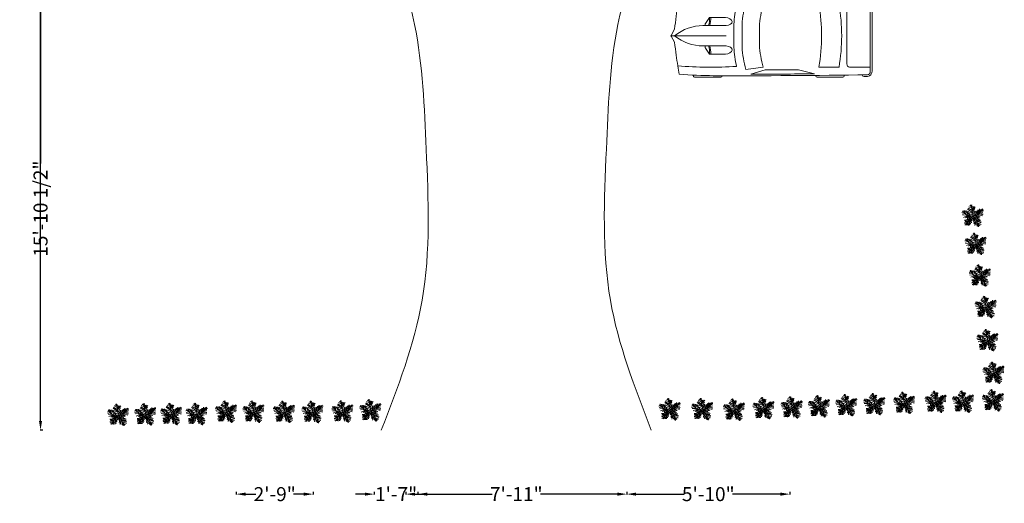
# Model space of a CAD drawing. Units: inches. Extents: x -81 to 380, y -521 to 79.
# Tile 1 of 5: x -81 to 342, y -521 to -313. Entities that reach past the tile are written whole.
import ezdxf

# ---------------------------------------------------------------- set-up
doc = ezdxf.new("R2010")
doc.units = ezdxf.units.IN
doc.header["$MEASUREMENT"] = 0
for name, color, linetype, lineweight in [('A-ANNO-DIMS', 2, 'Continuous', 18), ('C-ROAD-DRWY', 6, 'Continuous', 18), ('car', 33, 'Continuous', 18), ('trees', 3, 'Continuous', 13)]:
    doc.layers.add(name, color=color, linetype=linetype, lineweight=lineweight)
doc.styles.get("Standard").update_dxf_attribs({"font": 'arial.ttf'})
doc.dimstyles.get("Standard").update_dxf_attribs({"dimtxt": 6, "dimasz": 4, "dimexe": 0.18, "dimexo": 0.0625, "dimgap": 0.09, "dimtad": 0, "dimdec": 0, "dimzin": 0, "dimdsep": 46, "dimlunit": 3, "dimtxsty": 'Standard', "dimcen": 0.09, "dimclrd": 6, "dimclre": 6, "dimclrt": 2, "dimadec": 0, "dimazin": 0, "dimtfac": 1, "dimtdec": 0, "dimtofl": 0, "dimtmove": 0, "dimatfit": 3, "dimfxl": 1, "dimfxlon": 1, "dimtolj": 1, "dimtzin": 0, "dimarcsym": 0})

# ---------------------------------------------------------------- blocks, each defined once
blk = doc.blocks.new('*U4')
for p, q in [((-8.737, 47.138), (-17.069, 52.711)), ((-10.186, 53.64), (-13.084, 55.962)), ((0, 0), (-10.5, 57)), ((-9.099, 51.782), (-6.563, 55.962)), ((-7.65, 43.423), (-2.578, 49.46)), ((-47.498, 19.737), (-55.83, 18.344)), ((-40.615, 13.7), (-55.105, 10.913)), ((-31.5, 4.5), (-52.5, 25.5)), ((-33.37, 6.269), (-52.207, 5.34)), ((-48.585, 21.131), (-49.309, 29.026)), ((-28.299, 3.483), (-47.86, -5.805)), ((-43.513, 28.561), (-42.427, 15.558)), ((-38.442, 26.239), (-34.819, 7.663)), ((-21.416, 3.018), (-38.079, -8.128)), ((-35.544, 28.097), (-24.314, 3.947)), ((0, 0), (-31.5, 4.5)), ((-14.533, 2.09), (-30.834, 25.31)), ((-15.982, 2.09), (-30.11, -9.521)), ((-3.665, 19.273), (-27.574, 35.527)), ((-5.114, 28.097), (-24.676, 40.636)), ((-24.314, 23.917), (-2.941, 13.7)), ((0, 0), (-22.5, -19.5)), ((-7.288, 39.707), (-21.778, 46.673)), ((-6.563, 1.161), (-21.416, -8.128)), ((-20.691, 13.7), (-1.129, 4.876)), ((-5.839, 35.992), (4.667, 48.067)), ((-5.114, 27.632), (10.463, 46.673)), ((-2.941, 16.486), (8.652, 37.85)), ((-1.129, 6.734), (9.014, 26.704)), ((0, 0), (27, 9)), ((0, 0), (18, -22.5)), ((3.942, 1.625), (11.187, 24.381)), ((6.478, 1.625), (26.04, -8.592)), ((10.101, 3.483), (17.708, 26.239)), ((11.187, 3.483), (30.749, -5.805)), ((16.259, 5.805), (23.142, 31.348)), ((18.07, 5.805), (35.096, -3.483)), ((22.055, 7.198), (27.489, 32.277)), ((24.229, 7.663), (46.688, 1.625)), ((27, 9), (48, 36)), ((27.127, 9.056), (31.112, 35.992)), ((29.662, 12.307), (48.137, 6.269)), ((31.836, 30.883), (32.561, 16.486)), ((33.285, 16.486), (48.862, 10.913)), ((35.096, 32.741), (37.27, 22.524)), ((36.183, 19.737), (48.137, 17.88)), ((38.719, 34.134), (41.979, 28.561)), ((40.53, 25.775), (48.862, 24.846)), ((43.791, 29.954), (51.036, 30.883)), ((44.153, 36.456), (45.239, 32.741)), ((-17.431, -15.094), (-42.789, -18.809)), ((-28.299, -29.026), (-42.789, -31.348)), ((-24.314, -21.596), (-42.427, -22.06)), ((-30.834, -34.135), (-42.427, -35.528)), ((-34.457, -39.708), (-40.978, -42.494)), ((-26.849, -26.24), (-40.253, -25.775)), ((-22.5, -19.5), (-37.5, -45)), ((-32.646, -36.921), (-31.921, -44.352)), ((-15.257, -12.772), (-30.11, -12.772)), ((-29.023, -30.884), (-27.936, -43.887)), ((-25.038, -23.918), (-22.865, -45.281)), ((-20.691, -18.345), (-17.793, -44.352)), ((-6.563, -5.805), (-19.967, -9.985)), ((-17.069, -15.094), (-12.721, -40.172)), ((-13.446, -11.378), (-8.737, -32.741)), ((-9.461, -8.592), (-6.201, -23.453)), ((-4.752, -3.483), (-3.665, -14.629)), ((2.493, -3.019), (-1.491, -20.202)), ((1.769, -2.555), (24.229, -9.521)), ((5.029, -6.27), (2.131, -25.775)), ((9.014, -11.378), (3.58, -35.992)), ((14.085, -16.951), (6.478, -40.172)), ((7.565, -9.056), (32.198, -14.629)), ((18.07, -22.524), (8.289, -45.745)), ((12.274, -15.094), (36.907, -18.809)), ((20.244, -30.419), (15.897, -44.816)), ((16.259, -19.738), (36.183, -22.989)), ((18, -22.5), (27, -52.5)), ((18.433, -22.524), (40.53, -29.026)), ((19.157, -25.311), (38.719, -33.206)), ((22.78, -37.85), (19.519, -48.532)), ((21.331, -32.741), (39.081, -40.636)), ((22.78, -38.314), (34.372, -44.816)), ((24.591, -45.745), (23.142, -50.854)), ((24.591, -43.423), (30.749, -47.603)), ((26.764, -49.925), (28.213, -50.854))]:
    blk.add_line(p, q)
blk = doc.blocks.new('*U33')
for p, q in [((21.1, 37.41), (21.1, 36.83)), ((46.55, 38.89), (22.35, 38.89)), ((47.8, 37.39), (47.8, 37.41)), ((135.45, 37.07), (135.45, 37.41)), ((136.7, 38.89), (160.9, 38.89)), ((162.15, 37.41), (162.15, 36.77)), ((70.03, 31.54), (86.41, 29.35)), ((87.99, 31.87), (74.76, 35.92)), ((134.31, 35.6), (119.29, 31.78)), ((138.42, 29.35), (157.25, 29.35)), ((186.47, 29.35), (167.01, 29.35)), ((186.47, -33.5), (186.47, 33.5)), ((188.4, -32.76), (188.4, 32.76)), ((164.52, 26.39), (164.52, -26.39)), ((29.77, 9.51), (51.68, 9.51)), ((32.12, 9.51), (32.12, 11.15)), ((32.27, 11.63), (36.13, 17.17)), ((36.13, 17.17), (50.94, 17.17)), ((58.92, -10.77), (58.92, 10.77)), ((66.55, -10.53), (66.55, 10.53)), ((186.47, -10.53), (186.47, 10.53)), ((3.27, 6.13), (0.1, 0.41)), ((82.74, 8.5), (82.74, -8.5)), ((0, 0), (51.68, 0)), ((0.1, -0.41), (3.27, -6.13)), ((29.77, -9.51), (51.68, -9.51)), ((32.12, -9.51), (32.12, -11.15)), ((32.27, -11.63), (36.13, -17.17)), ((36.13, -17.17), (50.94, -17.17)), ((21.1, -37.41), (21.1, -36.83)), ((86.41, -29.35), (70.03, -31.54)), ((87.99, -31.87), (74.76, -35.92)), ((134.31, -35.6), (119.29, -31.78)), ((157.25, -29.35), (138.42, -29.35)), ((162.15, -37.41), (162.15, -36.77)), ((167.01, -29.35), (186.47, -29.35)), ((46.55, -38.89), (22.35, -38.89)), ((47.8, -37.39), (47.8, -37.41)), ((135.45, -37.07), (135.45, -37.41)), ((136.7, -38.89), (160.9, -38.89))]:
    blk.add_line(p, q)
for centre, major_axis, ratio, start_param, end_param in [((41.19, -490.86), (0, 528.23), 0.842304, 0.00281, 0.075598), ((22.35, 37.41), (0, -1.48), 0.842304, 3.141593, 4.712389), ((64.48, -10555.62), (0, 10593.03), 0.842304, -0.013397, 0.002797), ((46.55, 37.41), (0, 1.48), 0.842304, -1.570796, 0), ((136.7, 37.41), (0, -1.48), 0.842304, 3.141593, 4.712389), ((160.9, 37.41), (0, 1.48), 0.842304, -1.570796, 0), ((180.63, 35.84), (0, 2.22), 0.842304, -0.013017, 1.249894), ((64.48, -10556.36), (0, 10595.31), 0.842304, -0.013397, -0.013017), ((183.98, 32.76), (0, -5.25), 0.842304, 1.570796, 3.128196), ((259.18, -27.52), (0, -305.3), 0.842304, 4.528606, 4.561838), ((266.03, -27.52), (0, 313.31), 0.842304, 1.367076, 1.39176), ((37.47, -593.96), (0, -623.33), 0.842304, 3.096046, 3.200911), ((134.4, 5.39), (0, -89.78), 0.842304, 4.449482, 4.652344), ((135.29, 5.39), (0, 81.77), 0.842304, 1.245306, 1.50788), ((64.48, -10555.62), (0, -10591.55), 0.842304, 3.133765, 3.140441), ((149.6, 2.8), (0, -79.58), 0.842304, 4.372215, 4.640744), ((95.79, -3666.35), (0, -3698.24), 0.842304, 3.134049, 3.144098), ((17.08, 0), (0, 147.02), 0.842304, 4.511394, 4.913384), ((35.91, 0), (0, 147.02), 0.842304, 4.511394, 4.913384), ((167.01, 26.39), (0, 2.96), 0.842304, 0, 1.570796), ((183.98, 33.5), (0, -2.96), 0.842304, 1.570796, 3.128196), ((-204.49, 52.4), (0, -250.96), 0.842304, 1.385369, 1.434372), ((29.77, -46.66), (0, 56.17), 0.842304, 0, 0.590319), ((32.75, 11.15), (0, 0.74), 0.842304, 0.879714, 1.570796), ((13.04, 17.01), (0, 27.42), 0.842304, 4.435146, 4.718221), ((14.2, 17.01), (0, 27.42), 0.842304, 4.435146, 4.718221), ((50.79, 13.34), (6.34, -0.36), 0.603834, -1.395552, 1.581315), ((0.62, 0), (0, -0.74), 0.842304, 4.131459, 5.293319), ((-204.49, -52.4), (0, 250.96), 0.842304, -1.434372, -1.385369), ((29.77, 46.66), (0, 56.17), 0.842304, 2.551274, 3.141593), ((149.6, -2.8), (0, -79.58), 0.842304, -1.499151, -1.230623), ((259.18, 27.52), (0, 305.3), 0.842304, 1.721348, 1.754579), ((32.75, -11.15), (0, -0.74), 0.842304, 4.712389, 5.403472), ((13.04, -17.01), (0, -27.42), 0.842304, 1.564964, 1.848039), ((14.2, -17.01), (0, -27.42), 0.842304, 1.564964, 1.848039), ((134.4, -5.39), (0, -89.78), 0.842304, -1.510751, -1.307889), ((135.29, -5.39), (0, -81.77), 0.842304, -1.50788, -1.245306), ((167.01, -26.39), (0, -2.96), 0.842304, 4.712389, 6.283185), ((266.03, 27.52), (0, 313.31), 0.842304, 1.749832, 1.774517), ((37.47, 593.96), (0, -623.33), 0.842304, -0.059319, 0.045547), ((41.19, 490.86), (0, -528.23), 0.842304, -0.075598, -0.00281), ((64.48, 10555.62), (0, 10593.03), 0.842304, 3.138796, 3.15499), ((64.48, 10555.62), (0, -10591.55), 0.842304, 0.001152, 0.007828), ((95.79, 3666.35), (0, -3698.24), 0.842304, -0.002505, 0.007544), ((180.63, -35.84), (0, -2.22), 0.842304, -1.249894, 0.013017), ((183.98, -33.5), (0, 2.96), 0.842304, 3.15499, 4.712389), ((183.98, -32.76), (0, -5.25), 0.842304, 0.013397, 1.570796), ((22.35, -37.41), (0, 1.48), 0.842304, 1.570796, 3.141593), ((46.55, -37.41), (0, -1.48), 0.842304, 0, 1.570796), ((136.7, -37.41), (0, -1.48), 0.842304, -1.570796, 0), ((160.9, -37.41), (0, 1.48), 0.842304, 3.141593, 4.712389), ((64.48, 10556.36), (0, 10595.31), 0.842304, 3.15461, 3.15499)]:
    blk.add_ellipse(centre, major_axis=major_axis, ratio=ratio, start_param=start_param, end_param=end_param)
at = {"extrusion": (0, 0, -1)}
blk.add_ellipse((50.79, -13.34), major_axis=(6.34, 0.36), ratio=0.603834, start_param=-1.395552, end_param=1.581315, dxfattribs=at)
blk = doc.blocks.new('*D46')
at = {"layer": 'A-ANNO-DIMS', "color": 6, "lineweight": -2, "transparency": 16777216}
for p, q in [((74.55, 54.93), (74.55, 56.11)), ((78.55, 55.93), (124.45, 55.93)), ((186.48, 55.93), (140.58, 55.93)), ((190.48, 54.93), (190.48, 56.11))]:
    blk.add_line(p, q, dxfattribs=at)
at = {"layer": 'A-ANNO-DIMS', "color": 6, "transparency": 16777216}
for points in [[(78.55, 56.6), (78.55, 55.26), (74.55, 55.93)], [(186.48, 56.6), (186.48, 55.26), (190.48, 55.93)]]:
    blk.add_solid(points, dxfattribs=at)
at = {"layer": 'Defpoints', "color": 0, "transparency": 16777216}
for p in [(190.48, 55.93), (74.55, -489.67), (190.48, -489.67)]:
    blk.add_point(p, dxfattribs=at)
at = {"layer": 'A-ANNO-DIMS', "color": 2, "transparency": 16777216, "insert": (132.51, 55.93), "char_height": 6, "attachment_point": 5}
blk.add_mtext('\\A1;9\'-8"', dxfattribs=at)
blk = doc.blocks.new('*D47')
at = {"layer": 'A-ANNO-DIMS', "color": 6, "lineweight": -2, "transparency": 16777216}
for p, q in [((-70.72, -299.41), (-71.9, -299.41)), ((-71.72, -303.41), (-71.72, -375.11)), ((-71.72, -485.67), (-71.72, -413.98)), ((-70.72, -489.67), (-71.9, -489.67))]:
    blk.add_line(p, q, dxfattribs=at)
at = {"layer": 'A-ANNO-DIMS', "color": 6, "transparency": 16777216}
for points in [[(-72.39, -303.41), (-71.06, -303.41), (-71.72, -299.41)], [(-72.39, -485.67), (-71.06, -485.67), (-71.72, -489.67)]]:
    blk.add_solid(points, dxfattribs=at)
at = {"layer": 'Defpoints', "color": 0, "transparency": 16777216}
for p in [(-71.72, -299.41), (85.08, -299.41), (74.55, -489.67)]:
    blk.add_point(p, dxfattribs=at)
at = {"layer": 'A-ANNO-DIMS', "color": 2, "transparency": 16777216, "insert": (-71.72, -394.54), "char_height": 6, "attachment_point": 5, "rotation": 90}
blk.add_mtext('\\A1;15\'-10 1/2"', dxfattribs=at)
blk = doc.blocks.new('*D48')
at = {"layer": 'A-ANNO-DIMS', "color": 6, "lineweight": -2, "transparency": 16777216}
for p, q in [((-70.72, 28.48), (-71.9, 28.48)), ((-71.72, 24.48), (-71.72, -220.08)), ((-71.72, -485.67), (-71.72, -241.11)), ((-70.72, -489.67), (-71.9, -489.67))]:
    blk.add_line(p, q, dxfattribs=at)
at = {"layer": 'A-ANNO-DIMS', "color": 6, "transparency": 16777216}
for points in [[(-72.39, 24.48), (-71.06, 24.48), (-71.72, 28.48)], [(-72.39, -485.67), (-71.06, -485.67), (-71.72, -489.67)]]:
    blk.add_solid(points, dxfattribs=at)
at = {"layer": 'Defpoints', "color": 0, "transparency": 16777216}
for p in [(3.31, 28.48), (-71.72, -489.67), (74.55, -489.67)]:
    blk.add_point(p, dxfattribs=at)
at = {"layer": 'A-ANNO-DIMS', "color": 2, "transparency": 16777216, "insert": (-71.72, -230.6), "char_height": 6, "attachment_point": 5, "rotation": 90}
blk.add_mtext('\\A1;43\'-2"', dxfattribs=at)
blk = doc.blocks.new('*D49')
at = {"layer": 'A-ANNO-DIMS', "color": 6, "lineweight": -2, "transparency": 16777216}
for p, q in [((85.08, -516.12), (85.08, -517.3)), ((89.08, -517.12), (122.14, -517.12)), ((175.94, -517.12), (142.88, -517.12)), ((179.94, -516.12), (179.94, -517.3))]:
    blk.add_line(p, q, dxfattribs=at)
at = {"layer": 'A-ANNO-DIMS', "color": 6, "transparency": 16777216}
for points in [[(89.08, -516.45), (89.08, -517.79), (85.08, -517.12)], [(175.94, -516.45), (175.94, -517.79), (179.94, -517.12)]]:
    blk.add_solid(points, dxfattribs=at)
at = {"layer": 'Defpoints', "color": 0, "transparency": 16777216}
for p in [(85.08, -299.41), (179.94, -299.41), (179.94, -517.12)]:
    blk.add_point(p, dxfattribs=at)
at = {"layer": 'A-ANNO-DIMS', "color": 2, "transparency": 16777216, "insert": (132.51, -517.12), "char_height": 6, "attachment_point": 5}
blk.add_mtext('\\A1;7\'-11"', dxfattribs=at)
blk = doc.blocks.new('*D52')
at = {"layer": 'A-ANNO-DIMS', "color": 6, "lineweight": -2, "transparency": 16777216}
for p, q in [((179.94, -516.12), (179.94, -517.3)), ((183.94, -517.12), (204.55, -517.12)), ((245.94, -517.12), (225.34, -517.12)), ((249.94, -516.12), (249.94, -517.3))]:
    blk.add_line(p, q, dxfattribs=at)
at = {"layer": 'A-ANNO-DIMS', "color": 6, "transparency": 16777216}
for points in [[(183.94, -516.45), (183.94, -517.79), (179.94, -517.12)], [(245.94, -516.45), (245.94, -517.79), (249.94, -517.12)]]:
    blk.add_solid(points, dxfattribs=at)
at = {"layer": 'Defpoints', "color": 0, "transparency": 16777216}
for p in [(179.94, -292.11), (249.94, -292.11), (249.94, -517.12)]:
    blk.add_point(p, dxfattribs=at)
at = {"layer": 'A-ANNO-DIMS', "color": 2, "transparency": 16777216, "insert": (214.94, -517.12), "char_height": 6, "attachment_point": 5}
blk.add_mtext('\\A1;5\'-10"', dxfattribs=at)
blk = doc.blocks.new('*D55')
at = {"layer": 'A-ANNO-DIMS', "color": 6, "lineweight": -2, "transparency": 16777216}
for p, q in [((67.53, -517.12), (63.53, -517.12)), ((71.53, -516.12), (71.53, -517.3)), ((90.31, -516.12), (90.31, -517.3)), ((94.31, -517.12), (98.31, -517.12))]:
    blk.add_line(p, q, dxfattribs=at)
at = {"layer": 'A-ANNO-DIMS', "color": 6, "transparency": 16777216}
for points in [[(67.53, -516.45), (67.53, -517.79), (71.53, -517.12)], [(94.31, -516.45), (94.31, -517.79), (90.31, -517.12)]]:
    blk.add_solid(points, dxfattribs=at)
at = {"layer": 'Defpoints', "color": 0, "transparency": 16777216}
for p in [(71.53, -31.92), (90.31, -40.92), (90.31, -517.12)]:
    blk.add_point(p, dxfattribs=at)
at = {"layer": 'A-ANNO-DIMS', "color": 2, "transparency": 16777216, "insert": (80.92, -517.12), "char_height": 6, "attachment_point": 5}
blk.add_mtext('\\A1;1\'-7"', dxfattribs=at)
blk = doc.blocks.new('*D58')
at = {"layer": 'A-ANNO-DIMS', "color": 6, "lineweight": -2, "transparency": 16777216}
for p, q in [((12.31, -516.12), (12.31, -517.3)), ((16.31, -517.12), (20.69, -517.12)), ((41.3, -517.12), (36.92, -517.12)), ((45.3, -516.12), (45.3, -517.3))]:
    blk.add_line(p, q, dxfattribs=at)
at = {"layer": 'A-ANNO-DIMS', "color": 6, "transparency": 16777216}
for points in [[(16.31, -516.45), (16.31, -517.79), (12.31, -517.12)], [(41.3, -516.45), (41.3, -517.79), (45.3, -517.12)]]:
    blk.add_solid(points, dxfattribs=at)
at = {"layer": 'Defpoints', "color": 0, "transparency": 16777216}
for p in [(12.31, -100.52), (45.3, -100.52), (45.3, -517.12)]:
    blk.add_point(p, dxfattribs=at)
at = {"layer": 'A-ANNO-DIMS', "color": 2, "transparency": 16777216, "insert": (28.81, -517.12), "char_height": 6, "attachment_point": 5}
blk.add_mtext('\\A1;2\'-9"', dxfattribs=at)

msp = doc.modelspace()

# ---------------------------------------------------------------- linework, layer by layer
at = {"layer": 'C-ROAD-DRWY'}
for points in [[(85.08, -299.41), (86.43, -304.77), (92.17, -327.51), (93.95, -372.63), (96.69, -432.53), (81.67, -471.31), (74.55, -489.67)], [(179.94, -299.41), (178.59, -304.77), (172.86, -327.51), (171.08, -372.63), (168.34, -432.53), (183.36, -471.31), (190.48, -489.67)]]:
    msp.add_open_spline(points, degree=3, knots=[0, 0, 0, 0, 16.553876, 70.232148, 135.187628, 193.647877, 193.647877, 193.647877, 193.647877], dxfattribs=at)

# ---------------------------------------------------------------- block references
at = {"layer": 'car', "xscale": 0.4587568616370848, "yscale": 0.4587568616370848, "zscale": 0.4587568616370848}
msp.add_blockref('*U33', (198.93, -320.32), dxfattribs=at)
at = {"layer": 'trees', "xscale": 0.0864443764377546, "yscale": 0.0864443764377546, "zscale": 0.0864443764377546}
for p in [(328.66, -397.8), (329.92, -409.9), (331.73, -423.5), (334.26, -436.99), (334.99, -451.23), (337.61, -465.23), (299.23, -478.16), (312.75, -477.69), (324.53, -477.64), (337.35, -477.05), (8.13, -481.94), (19.91, -481.92), (33.03, -482), (45.22, -482.05), (58.09, -481.88), (70.1, -481.36), (198.6, -480.91), (212.54, -480.87), (226.17, -481.09), (238.87, -480.46), (250.97, -480.11), (262.64, -479.64), (274.41, -479.17), (286.42, -478.71), (-38.21, -483.31), (-26.58, -483.09), (-15.45, -482.92), (-4.51, -482.96)]:
    msp.add_blockref('*U4', p, dxfattribs=at)

# ---------------------------------------------------------------- dimensions: what is measured, and where the dimension line sits
at = {"layer": 'A-ANNO-DIMS'}
for base, p1, p2, picture, middle in [((190.48, 55.93), (74.55, -489.67), (190.48, -489.67), '*D46', (132.51, 55.93)), ((90.31, -517.12), (71.53, -31.92), (90.31, -40.92), '*D55', (80.92, -517.12)), ((45.3, -517.12), (12.31, -100.52), (45.3, -100.52), '*D58', (28.81, -517.12)), ((249.94, -517.12), (179.94, -292.11), (249.94, -292.11), '*D52', (214.94, -517.12)), ((179.94, -517.12), (85.08, -299.41), (179.94, -299.41), '*D49', (132.51, -517.12))]:
    dim = msp.add_linear_dim(base=base, p1=p1, p2=p2, dimstyle='Standard', override={"dimdec": 1, "dimlfac": 1, "dimrnd": 0, "dimzin": 1, "dimdsep": 46, "dimlunit": 4, "dimfrac": 2}, dxfattribs=at)
    dim.commit()
    dim.dimension.update_dxf_attribs({"geometry": picture, "text_midpoint": middle})
for base, p1, p2, picture, middle in [((-71.7227, -489.6708), (3.3113, 28.4806), (74.5527, -489.6708), '*D48', (-71.7227, -230.5951)), ((-71.72, -299.41), (74.55, -489.67), (85.08, -299.41), '*D47', (-71.72, -394.54))]:
    dim = msp.add_linear_dim(base=base, p1=p1, p2=p2, angle=90, dimstyle='Standard', override={"dimdec": 1, "dimlfac": 1, "dimrnd": 0, "dimzin": 1, "dimdsep": 46, "dimlunit": 4, "dimfrac": 2}, dxfattribs=at)
    dim.commit()
    dim.dimension.update_dxf_attribs({"geometry": picture, "text_midpoint": middle})

doc.saveas('drawing.dxf')
